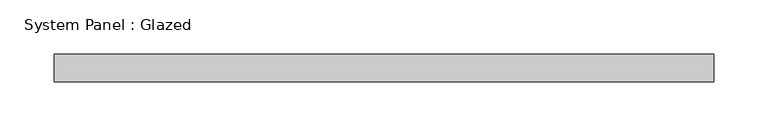
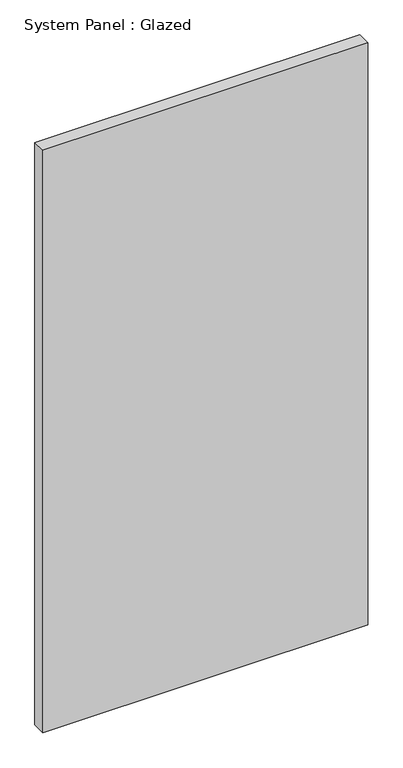
"""IFC4 building model written with IfcOpenShell, lengths in millimetres: plate geometry, System Panel : Glazed."""

from ifc_helpers import new_model, si_unit, origin, origin_with_axes, place, context, project, spatial, polyline, outline, extrude, source, transform, mapped, element, save


def system_panel_glazed_7af1c9c3(model_context):
    return source(origin(), model_context, "Body", "SweptSolid", [
        extrude(outline(polyline([(304.8, 19.05), (-304.8, 19.05), (-304.8, 44.45), (304.8, 44.45), (304.8, 19.05)])), origin_with_axes(), (0.0, 0.0, 1.0), 1155.7),
    ])


if __name__ == "__main__":
    model = new_model("IFC4")
    model_context = context("Model", 3, world=origin())
    ifc_project = project(units=[si_unit("LENGTHUNIT", "METRE", prefix="MILLI")], contexts=[model_context])
    site = spatial("IfcSite", under=ifc_project)
    building = spatial("IfcBuilding", under=site)
    placement = place(None, origin())
    system_panel_glazed_shape = system_panel_glazed_7af1c9c3(model_context)
    element("IfcPlate", 1, ObjectType="System Panel : Glazed", at=placement, inside=building, context=model_context, shape_type="MappedRepresentation", body=[
        mapped(system_panel_glazed_shape, transform((0.0, 0.0, 0.0), x_axis=(1.0, 0.0, 0.0), y_axis=(0.0, 1.0, 0.0), z_axis=(0.0, 0.0, 1.0))),
    ])
    save(model, "model.ifc")

# Revit data of these elements
# Type "System Panel : Glazed"
#   Construction Type Id = "GSP4R"
#   Analytic Construction = "1/8 in Pilkington single glazing"
#   Visual Light Transmittance = 0.9
#   Solar Heat Gain Coefficient = 0.86
#   Heat Transfer Coefficient (U) = 1.18115 BTU/(h·ft²·°F)
# Element 1 (IfcPlate, "System Panel : Glazed")
#   Materials on its faces: "Glass"
# Materials
#   "Glass": class "Glass", colour RGB 0 128 192, transparency 0.75, Description = "Soda Lime Glass", Cost = 0
